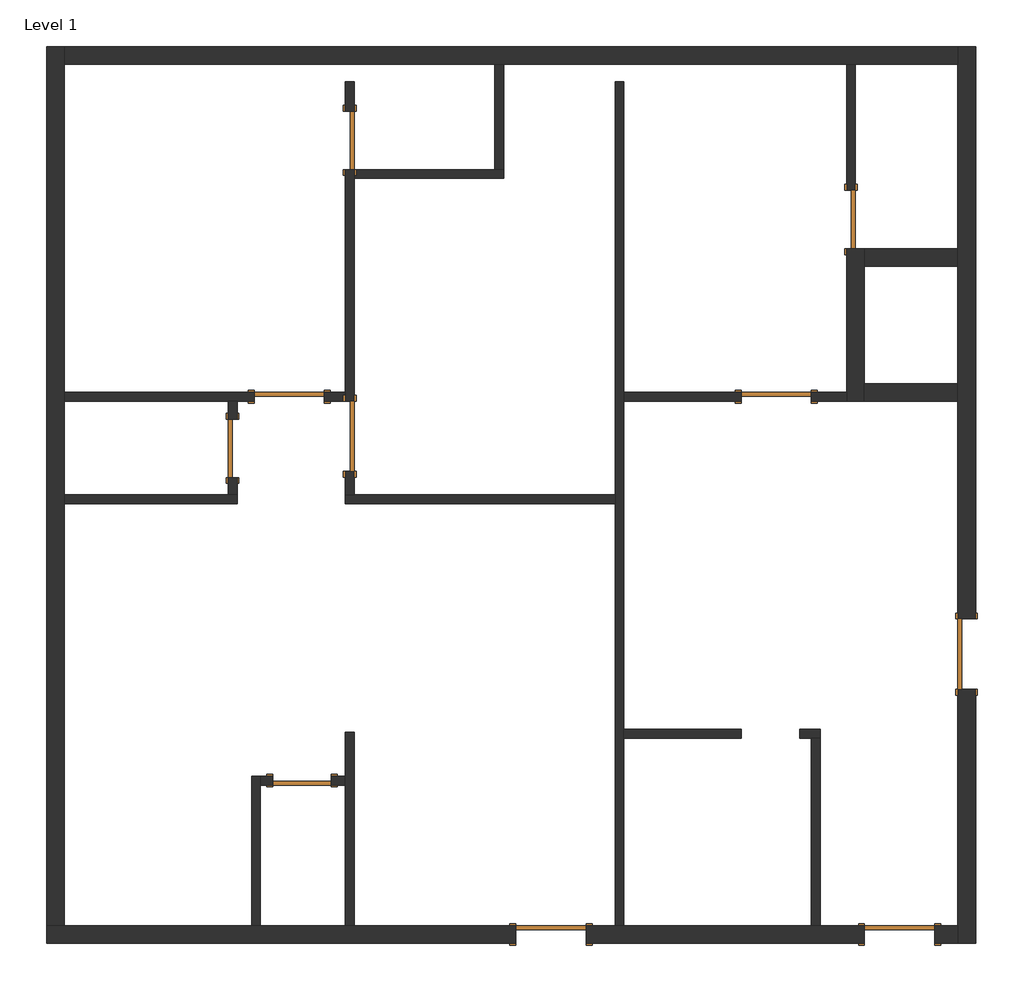
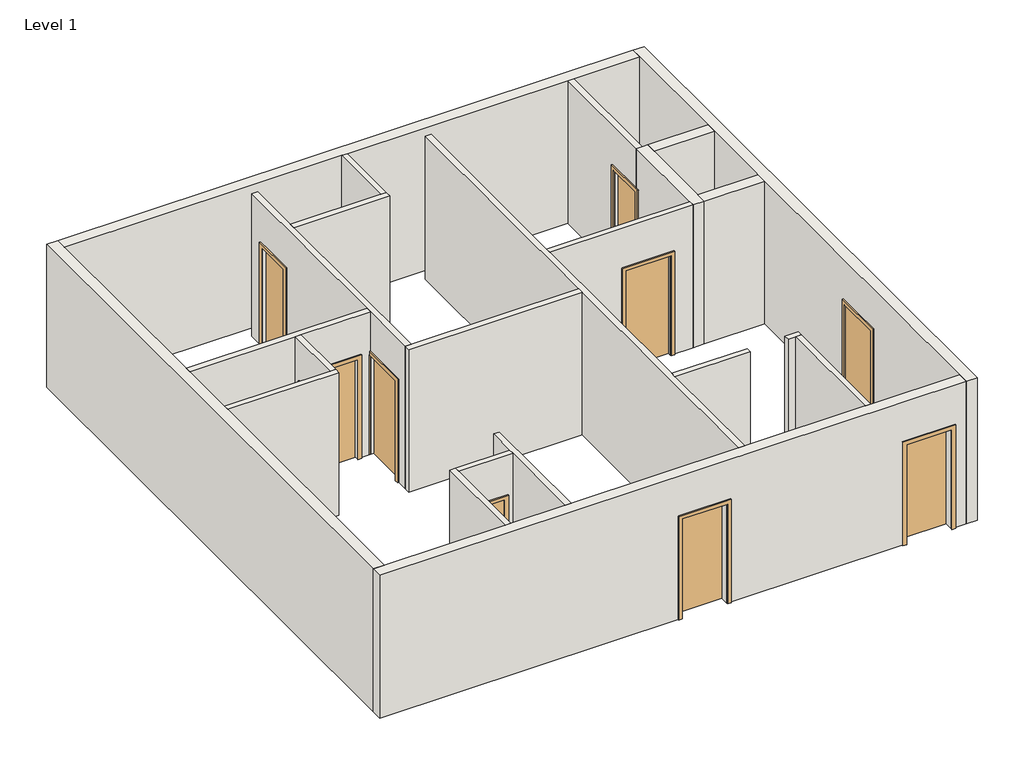
# One storey: 23 walls, 10 doors.
"""IFC4 building model written with IfcOpenShell, lengths in millimetres."""

from ifc_helpers import new_model, si_unit, frame, origin, origin_with_axes, place, context, project, spatial, polyline, outline, extrude, faceted_brep, transform, mapped, element, save
from components import door_214872d5, door_78caadf7, door_e5f9f3c4, door_0ca8825f, door_a90ba1ad

model = new_model("IFC4")

# Units and contexts
model_context = context("Model", 3, world=origin())
ifc_project = project(units=[si_unit("LENGTHUNIT", "METRE", prefix="MILLI")], contexts=[model_context])

# Site, building, storey
site = spatial("IfcSite", under=ifc_project)
building = spatial("IfcBuilding", under=site)
storey = spatial("IfcBuildingStorey", under=building, Name="Level 1", Elevation=0.0)

# Doors
placement = place(None, origin())
door_shape = door_214872d5(model_context)
element("IfcDoor", 1, ObjectType="Single-Flush : 30\" x 84\"", at=placement, inside=storey, context=model_context, shape_type="MappedRepresentation", body=[
    mapped(door_shape, transform((-4308.2802303, 5667.3877739, 0.0), x_axis=(0.0, -1.0, 0.0), y_axis=(1.0, 0.0, 0.0), z_axis=(0.0, 0.0, 1.0))),
])
element("IfcDoor", 2, ObjectType="Single-Flush : 30\" x 84\"", at=placement, inside=storey, context=model_context, shape_type="MappedRepresentation", body=[
    mapped(door_shape, transform((2206.8197697, 4638.6877739, 0.0), x_axis=(0.0, -1.0, 0.0), y_axis=(1.0, 0.0, 0.0), z_axis=(0.0, 0.0, 1.0))),
])
element("IfcDoor", 3, ObjectType="Single-Flush : 30\" x 84\"", at=placement, inside=storey, context=model_context, shape_type="MappedRepresentation", body=[
    mapped(door_shape, transform((-5832.2802303, 1662.8764801, 0.0), x_axis=(0.0, 1.0, 0.0), y_axis=(-1.0, 0.0, 0.0), z_axis=(0.0, 0.0, 1.0))),
])
door_2_shape = door_78caadf7(model_context)
element("IfcDoor", 4, ObjectType="Single-Flush : 30\" x 84\"", at=placement, inside=storey, context=model_context, shape_type="MappedRepresentation", body=[
    mapped(door_2_shape, transform((-4929.4173805, -2657.4622261, 0.0), x_axis=(1.0, 0.0, 0.0), y_axis=(0.0, 1.0, 0.0), z_axis=(0.0, 0.0, 1.0))),
])
door_3_shape = door_e5f9f3c4(model_context)
element("IfcDoor", 5, ObjectType="Single-Flush : 36\" x 84\"", at=placement, inside=storey, context=model_context, shape_type="MappedRepresentation", body=[
    mapped(door_3_shape, transform((-5096.3129519, 2333.6377739, 0.0), x_axis=(1.0, 0.0, 0.0), y_axis=(0.0, 1.0, 0.0), z_axis=(0.0, 0.0, 1.0))),
])
element("IfcDoor", 6, ObjectType="Single-Flush : 36\" x 84\"", at=placement, inside=storey, context=model_context, shape_type="MappedRepresentation", body=[
    mapped(door_3_shape, transform((-4308.2802303, 1819.2877739, 0.0), x_axis=(0.0, -1.0, 0.0), y_axis=(1.0, 0.0, 0.0), z_axis=(0.0, 0.0, 1.0))),
])
element("IfcDoor", 7, ObjectType="Single-Flush : 36\" x 84\"", at=placement, inside=storey, context=model_context, shape_type="MappedRepresentation", body=[
    mapped(door_3_shape, transform((1235.2697697, 2333.6377739, 0.0), x_axis=(1.0, 0.0, 0.0), y_axis=(0.0, 1.0, 0.0), z_axis=(0.0, 0.0, 1.0))),
])
door_4_shape = door_0ca8825f(model_context)
element("IfcDoor", 8, ObjectType="Single-Flush : 36\" x 84\"", at=placement, inside=storey, context=model_context, shape_type="MappedRepresentation", body=[
    mapped(door_4_shape, transform((2839.8620702, -4657.7122261, 0.0), x_axis=(1.0, 0.0, 0.0), y_axis=(0.0, 1.0, 0.0), z_axis=(0.0, 0.0, 1.0))),
])
element("IfcDoor", 9, ObjectType="Single-Flush : 36\" x 84\"", at=placement, inside=storey, context=model_context, shape_type="MappedRepresentation", body=[
    mapped(door_4_shape, transform((-1692.7716329, -4657.7122261, 0.0), x_axis=(1.0, 0.0, 0.0), y_axis=(0.0, 1.0, 0.0), z_axis=(0.0, 0.0, 1.0))),
])
door_5_shape = door_a90ba1ad(model_context)
element("IfcDoor", 10, ObjectType="Single-Flush : 36\" x 84\"", at=placement, inside=storey, context=model_context, shape_type="MappedRepresentation", body=[
    mapped(door_5_shape, transform((3711.7697697, -1012.8122261, 0.0), x_axis=(0.0, -1.0, 0.0), y_axis=(1.0, 0.0, 0.0), z_axis=(0.0, 0.0, 1.0))),
])

# Walls
element("IfcWall", 11, ObjectType="Generic - 4.5\"", at=placement, inside=storey, context=model_context, shape_type="Brep", body=[
    faceted_brep([(-4639.1129519, 2276.4877739, 2133.6), (-4639.1129519, 2276.4877739, 0.0), (-4365.4302303, 2276.4877739, 0.0), (-4365.4302303, 2276.4877739, 3048.0), (-5775.1302303, 2276.4877739, 3048.0), (-5889.4302303, 2276.4877739, 3048.0), (-8023.0302303, 2276.4877739, 3048.0), (-8023.0302303, 2276.4877739, 0.0), (-5889.4302303, 2276.4877739, 0.0), (-5775.1302303, 2276.4877739, 0.0), (-5553.5129519, 2276.4877739, 0.0), (-5553.5129519, 2276.4877739, 2133.6), (-4365.4302303, 2390.7877739, 0.0), (-4639.1129519, 2390.7877739, 0.0), (-4639.1129519, 2390.7877739, 2133.6), (-5553.5129519, 2390.7877739, 2133.6), (-5553.5129519, 2390.7877739, 0.0), (-8023.0302303, 2390.7877739, 0.0), (-8023.0302303, 2390.7877739, 3048.0), (-4365.4302303, 2390.7877739, 3048.0)], [[[0, 1, 2, 3, 4, 5, 6, 7, 8, 9, 10, 11]], [[12, 13, 14, 15, 16, 17, 18, 19]], [[2, 1, 13, 12]], [[10, 9, 8, 7, 17, 16]], [[6, 5, 4, 3, 19, 18]], [[7, 6, 18, 17]], [[3, 2, 12, 19]], [[14, 13, 1, 0]], [[15, 14, 0, 11]], [[16, 15, 11, 10]]]),
])
element("IfcWall", 12, ObjectType="Generic - 4.5\"", at=placement, inside=storey, context=model_context, shape_type="Brep", body=[
    faceted_brep([(-4251.1302303, 2276.4877739, 0.0), (-4251.1302303, 5172.0877739, 0.0), (-4251.1302303, 5286.3877739, 0.0), (-4251.1302303, 5286.3877739, 2133.6), (-4251.1302303, 6048.3877739, 2133.6), (-4251.1302303, 6048.3877739, 0.0), (-4251.1302303, 6429.3877739, 0.0), (-4251.1302303, 6429.3877739, 3048.0), (-4251.1302303, 5286.3877739, 3048.0), (-4251.1302303, 5172.0877739, 3048.0), (-4251.1302303, 1057.2877739, 3048.0), (-4251.1302303, 1057.2877739, 0.0), (-4251.1302303, 1362.0877739, 0.0), (-4251.1302303, 1362.0877739, 2133.6), (-4251.1302303, 2276.4877739, 2133.6), (-4365.4302303, 5286.3877739, 2133.6), (-4365.4302303, 5286.3877739, 0.0), (-4365.4302303, 2390.7877739, 0.0), (-4365.4302303, 2276.4877739, 0.0), (-4365.4302303, 2276.4877739, 2133.6), (-4365.4302303, 1362.0877739, 2133.6), (-4365.4302303, 1362.0877739, 0.0), (-4365.4302303, 1057.2877739, 0.0), (-4365.4302303, 1057.2877739, 3048.0), (-4365.4302303, 2276.4877739, 3048.0), (-4365.4302303, 2390.7877739, 3048.0), (-4365.4302303, 6429.3877739, 3048.0), (-4365.4302303, 6429.3877739, 0.0), (-4365.4302303, 6048.3877739, 0.0), (-4365.4302303, 6048.3877739, 2133.6)], [[[0, 1, 2, 3, 4, 5, 6, 7, 8, 9, 10, 11, 12, 13, 14]], [[15, 16, 17, 18, 19, 20, 21, 22, 23, 24, 25, 26, 27, 28, 29]], [[22, 21, 12, 11]], [[28, 27, 6, 5]], [[18, 17, 16, 2, 1, 0]], [[7, 6, 27, 26]], [[10, 9, 8, 7, 26, 25, 24, 23]], [[11, 10, 23, 22]], [[13, 12, 21, 20]], [[14, 13, 20, 19]], [[0, 14, 19, 18]], [[3, 2, 16, 15]], [[4, 3, 15, 29]], [[5, 4, 29, 28]]]),
])
element("IfcWall", 13, ObjectType="Generic - 4.5\"", at=placement, inside=storey, context=model_context, shape_type="Brep", body=[
    faceted_brep([(-4251.1302303, 5172.0877739, 0.0), (-2308.0302303, 5172.0877739, 0.0), (-2308.0302303, 5172.0877739, 3048.0), (-4251.1302303, 5172.0877739, 3048.0), (-4251.1302303, 5286.3877739, 0.0), (-4251.1302303, 5286.3877739, 3048.0), (-2422.3302303, 5286.3877739, 3048.0), (-2308.0302303, 5286.3877739, 3048.0), (-2308.0302303, 5286.3877739, 0.0), (-2422.3302303, 5286.3877739, 0.0)], [[[0, 1, 2, 3]], [[4, 5, 6, 7, 8, 9]], [[1, 0, 4, 9, 8]], [[3, 2, 7, 6, 5]], [[2, 1, 8, 7]], [[0, 3, 5, 4]]]),
])
element("IfcWall", 14, ObjectType="Generic - 4.5\"", at=placement, inside=storey, context=model_context, shape_type="SweptSolid", body=[
    extrude(outline(polyline([(-2308.0302303, 6657.9877739), (-2308.0302303, 5286.3877739), (-2422.3302303, 5286.3877739), (-2422.3302303, 6657.9877739), (-2308.0302303, 6657.9877739)])), origin_with_axes(), (0.0, 0.0, 1.0), 3048.0),
])
element("IfcWall", 15, ObjectType="Generic - 4.5\"", at=placement, inside=storey, context=model_context, shape_type="SweptSolid", body=[
    extrude(outline(polyline([(4257.6877739, 3048.0), (6657.9877739, 3048.0), (6657.9877739, 0.0), (5019.6877739, 0.0), (5019.6877739, 2133.6), (4257.6877739, 2133.6), (4257.6877739, 3048.0)])), frame((2149.6697697, 0.0, 0.0), z_axis=(1.0, 0.0, 0.0), x_axis=(0.0, 1.0, 0.0)), (0.0, 0.0, 1.0), 114.3),
])
element("IfcWall", 16, ObjectType="Generic - 4.5\"", at=placement, inside=storey, context=model_context, shape_type="Brep", body=[
    faceted_brep([(-5470.3302303, -4543.4122261, 0.0), (-5470.3302303, -2714.6122261, 0.0), (-5470.3302303, -2600.3122261, 0.0), (-5470.3302303, -2600.3122261, 3048.0), (-5470.3302303, -2714.6122261, 3048.0), (-5470.3302303, -4543.4122261, 3048.0), (-5584.6302303, -4543.4122261, 0.0), (-5584.6302303, -4543.4122261, 3048.0), (-5584.6302303, -2600.3122261, 3048.0), (-5584.6302303, -2600.3122261, 0.0)], [[[0, 1, 2, 3, 4, 5]], [[6, 7, 8, 9]], [[2, 1, 0, 6, 9]], [[5, 4, 3, 8, 7]], [[0, 5, 7, 6]], [[3, 2, 9, 8]]]),
])
element("IfcWall", 17, ObjectType="Generic - 4.5\"", at=placement, inside=storey, context=model_context, shape_type="SweptSolid", body=[
    extrude(outline(polyline([(2133.6, -4548.4173805), (0.0, -4548.4173805), (0.0, -4365.4302303), (3048.0, -4365.4302303), (3048.0, -5470.3302303), (0.0, -5470.3302303), (0.0, -5310.4173805), (2133.6, -5310.4173805), (2133.6, -4548.4173805)])), frame((0.0, -2714.6122261, 0.0), z_axis=(0.0, 1.0, 0.0), x_axis=(0.0, 0.0, 1.0)), (0.0, 0.0, 1.0), 114.3),
])
element("IfcWall", 18, ObjectType="Generic - 4.5\"", at=placement, inside=storey, context=model_context, shape_type="Brep", body=[
    faceted_brep([(-4251.1302303, -4543.4122261, 0.0), (-4251.1302303, -2028.8122261, 0.0), (-4251.1302303, -2028.8122261, 3048.0), (-4251.1302303, -4543.4122261, 3048.0), (-4365.4302303, -4543.4122261, 0.0), (-4365.4302303, -4543.4122261, 3048.0), (-4365.4302303, -2714.6122261, 3048.0), (-4365.4302303, -2600.3122261, 3048.0), (-4365.4302303, -2028.8122261, 3048.0), (-4365.4302303, -2028.8122261, 0.0), (-4365.4302303, -2600.3122261, 0.0), (-4365.4302303, -2714.6122261, 0.0)], [[[0, 1, 2, 3]], [[4, 5, 6, 7, 8, 9, 10, 11]], [[1, 0, 4, 11, 10, 9]], [[2, 1, 9, 8]], [[3, 2, 8, 7, 6, 5]], [[0, 3, 5, 4]]]),
])
element("IfcWall", 19, ObjectType="Generic - 4.5\"", at=placement, inside=storey, context=model_context, shape_type="Brep", body=[
    faceted_brep([(-745.9302303, -4543.4122261, 0.0), (-745.9302303, -2105.0122261, 0.0), (-745.9302303, -1990.7122261, 0.0), (-745.9302303, 2276.4877739, 0.0), (-745.9302303, 2390.7877739, 0.0), (-745.9302303, 6429.3877739, 0.0), (-745.9302303, 6429.3877739, 3048.0), (-745.9302303, 2390.7877739, 3048.0), (-745.9302303, 2276.4877739, 3048.0), (-745.9302303, -1990.7122261, 3048.0), (-745.9302303, -2105.0122261, 3048.0), (-745.9302303, -4543.4122261, 3048.0), (-860.2302303, -4543.4122261, 0.0), (-860.2302303, -4543.4122261, 3048.0), (-860.2302303, 942.9877739, 3048.0), (-860.2302303, 1057.2877739, 3048.0), (-860.2302303, 6429.3877739, 3048.0), (-860.2302303, 6429.3877739, 0.0), (-860.2302303, 1057.2877739, 0.0), (-860.2302303, 942.9877739, 0.0)], [[[0, 1, 2, 3, 4, 5, 6, 7, 8, 9, 10, 11]], [[12, 13, 14, 15, 16, 17, 18, 19]], [[5, 4, 3, 2, 1, 0, 12, 19, 18, 17]], [[6, 5, 17, 16]], [[11, 10, 9, 8, 7, 6, 16, 15, 14, 13]], [[0, 11, 13, 12]]]),
])
element("IfcWall", 20, ObjectType="Generic - 4.5\"", at=placement, inside=storey, context=model_context, shape_type="SweptSolid", body=[
    extrude(outline(polyline([(2133.6, 1692.4697697), (0.0, 1692.4697697), (0.0, 2149.6697697), (3048.0, 2149.6697697), (3048.0, -745.9302303), (0.0, -745.9302303), (0.0, 778.0697697), (2133.6, 778.0697697), (2133.6, 1692.4697697)])), frame((0.0, 2276.4877739, 0.0), z_axis=(0.0, 1.0, 0.0), x_axis=(0.0, 0.0, 1.0)), (0.0, 0.0, 1.0), 114.3),
])
element("IfcWall", 21, ObjectType="Generic - 4.5\"", at=placement, inside=storey, context=model_context, shape_type="Brep", body=[
    faceted_brep([(1540.0697697, -2105.0122261, 0.0), (1692.4697697, -2105.0122261, 0.0), (1806.7697697, -2105.0122261, 0.0), (1806.7697697, -2105.0122261, 3048.0), (1692.4697697, -2105.0122261, 3048.0), (1540.0697697, -2105.0122261, 3048.0), (1540.0697697, -1990.7122261, 0.0), (1540.0697697, -1990.7122261, 3048.0), (1806.7697697, -1990.7122261, 3048.0), (1806.7697697, -1990.7122261, 0.0)], [[[0, 1, 2, 3, 4, 5]], [[6, 7, 8, 9]], [[2, 1, 0, 6, 9]], [[5, 4, 3, 8, 7]], [[0, 5, 7, 6]], [[3, 2, 9, 8]]]),
])
element("IfcWall", 22, ObjectType="Generic - 4.5\"", at=placement, inside=storey, context=model_context, shape_type="SweptSolid", body=[
    extrude(outline(polyline([(1692.4697697, -4543.4122261), (1692.4697697, -2105.0122261), (1806.7697697, -2105.0122261), (1806.7697697, -4543.4122261), (1692.4697697, -4543.4122261)])), origin_with_axes(), (0.0, 0.0, 1.0), 3048.0),
])
element("IfcWall", 23, ObjectType="Generic - 4.5\"", at=placement, inside=storey, context=model_context, shape_type="SweptSolid", body=[
    extrude(outline(polyline([(-745.9302303, -1990.7122261), (778.0697697, -1990.7122261), (778.0697697, -2105.0122261), (-745.9302303, -2105.0122261), (-745.9302303, -1990.7122261)])), origin_with_axes(), (0.0, 0.0, 1.0), 3048.0),
])
element("IfcWall", 24, ObjectType="Generic - 4.5\"", at=placement, inside=storey, context=model_context, shape_type="Brep", body=[
    faceted_brep([(-860.2302303, 1057.2877739, 0.0), (-4251.1302303, 1057.2877739, 0.0), (-4365.4302303, 1057.2877739, 0.0), (-4365.4302303, 1057.2877739, 3048.0), (-4251.1302303, 1057.2877739, 3048.0), (-860.2302303, 1057.2877739, 3048.0), (-860.2302303, 942.9877739, 0.0), (-860.2302303, 942.9877739, 3048.0), (-4365.4302303, 942.9877739, 3048.0), (-4365.4302303, 942.9877739, 0.0)], [[[0, 1, 2, 3, 4, 5]], [[6, 7, 8, 9]], [[2, 1, 0, 6, 9]], [[3, 2, 9, 8]], [[5, 4, 3, 8, 7]], [[0, 5, 7, 6]]]),
])
element("IfcWall", 25, ObjectType="Generic - 4.5\"", at=placement, inside=storey, context=model_context, shape_type="Brep", body=[
    faceted_brep([(-8023.0302303, 942.9877739, 0.0), (-5775.1302303, 942.9877739, 0.0), (-5775.1302303, 942.9877739, 3048.0), (-8023.0302303, 942.9877739, 3048.0), (-8023.0302303, 1057.2877739, 0.0), (-8023.0302303, 1057.2877739, 3048.0), (-5889.4302303, 1057.2877739, 3048.0), (-5775.1302303, 1057.2877739, 3048.0), (-5775.1302303, 1057.2877739, 0.0), (-5889.4302303, 1057.2877739, 0.0)], [[[0, 1, 2, 3]], [[4, 5, 6, 7, 8, 9]], [[1, 0, 4, 9, 8]], [[3, 2, 7, 6, 5]], [[0, 3, 5, 4]], [[2, 1, 8, 7]]]),
])
element("IfcWall", 26, ObjectType="Generic - 4.5\"", at=placement, inside=storey, context=model_context, shape_type="SweptSolid", body=[
    extrude(outline(polyline([(2276.4877739, 0.0), (2043.8764801, 0.0), (2043.8764801, 2133.6), (1281.8764801, 2133.6), (1281.8764801, 0.0), (1057.2877739, 0.0), (1057.2877739, 3048.0), (2276.4877739, 3048.0), (2276.4877739, 0.0)])), frame((-5889.4302303, 0.0, 0.0), z_axis=(1.0, 0.0, 0.0), x_axis=(0.0, 1.0, 0.0)), (0.0, 0.0, 1.0), 114.3),
])
element("IfcWall", 27, ObjectType="Generic - 9\"", at=placement, inside=storey, context=model_context, shape_type="Brep", body=[
    faceted_brep([(3597.4697697, -1470.0122261, 2133.6), (3597.4697697, -1470.0122261, 0.0), (3597.4697697, -4543.4122261, 0.0), (3597.4697697, -4772.0122261, 0.0), (3597.4697697, -4772.0122261, 3048.0), (3597.4697697, -4543.4122261, 3048.0), (3597.4697697, 2276.4877739, 3048.0), (3597.4697697, 2505.0877739, 3048.0), (3597.4697697, 4029.0877739, 3048.0), (3597.4697697, 4257.6877739, 3048.0), (3597.4697697, 6657.9877739, 3048.0), (3597.4697697, 6886.5877739, 3048.0), (3597.4697697, 6886.5877739, 0.0), (3597.4697697, 6657.9877739, 0.0), (3597.4697697, 4257.6877739, 0.0), (3597.4697697, 4029.0877739, 0.0), (3597.4697697, 2505.0877739, 0.0), (3597.4697697, 2276.4877739, 0.0), (3597.4697697, -555.6122261, 0.0), (3597.4697697, -555.6122261, 2133.6), (3826.0697697, -4772.0122261, 0.0), (3826.0697697, -1470.0122261, 0.0), (3826.0697697, -1470.0122261, 2133.6), (3826.0697697, -555.6122261, 2133.6), (3826.0697697, -555.6122261, 0.0), (3826.0697697, 6886.5877739, 0.0), (3826.0697697, 6886.5877739, 3048.0), (3826.0697697, -4772.0122261, 3048.0)], [[[0, 1, 2, 3, 4, 5, 6, 7, 8, 9, 10, 11, 12, 13, 14, 15, 16, 17, 18, 19]], [[20, 21, 22, 23, 24, 25, 26, 27]], [[3, 2, 1, 21, 20]], [[18, 17, 16, 15, 14, 13, 12, 25, 24]], [[11, 10, 9, 8, 7, 6, 5, 4, 27, 26]], [[4, 3, 20, 27]], [[12, 11, 26, 25]], [[22, 21, 1, 0]], [[23, 22, 0, 19]], [[24, 23, 19, 18]]]),
])
element("IfcWall", 28, ObjectType="Generic - 9\"", at=placement, inside=storey, context=model_context, shape_type="Brep", body=[
    faceted_brep([(2382.6620702, -4543.4122261, 0.0), (1806.7697697, -4543.4122261, 0.0), (1692.4697697, -4543.4122261, 0.0), (-745.9302303, -4543.4122261, 0.0), (-860.2302303, -4543.4122261, 0.0), (-1235.5716329, -4543.4122261, 0.0), (-1235.5716329, -4543.4122261, 2133.6), (-2149.9716329, -4543.4122261, 2133.6), (-2149.9716329, -4543.4122261, 0.0), (-4251.1302303, -4543.4122261, 0.0), (-4365.4302303, -4543.4122261, 0.0), (-5470.3302303, -4543.4122261, 0.0), (-5584.6302303, -4543.4122261, 0.0), (-8023.0302303, -4543.4122261, 0.0), (-8251.6302303, -4543.4122261, 0.0), (-8251.6302303, -4543.4122261, 3048.0), (-8023.0302303, -4543.4122261, 3048.0), (-5584.6302303, -4543.4122261, 3048.0), (-5470.3302303, -4543.4122261, 3048.0), (-4365.4302303, -4543.4122261, 3048.0), (-4251.1302303, -4543.4122261, 3048.0), (-860.2302303, -4543.4122261, 3048.0), (-745.9302303, -4543.4122261, 3048.0), (1692.4697697, -4543.4122261, 3048.0), (1806.7697697, -4543.4122261, 3048.0), (3597.4697697, -4543.4122261, 3048.0), (3597.4697697, -4543.4122261, 0.0), (3297.0620702, -4543.4122261, 0.0), (3297.0620702, -4543.4122261, 2133.6), (2382.6620702, -4543.4122261, 2133.6), (-1235.5716329, -4772.0122261, 2133.6), (-1235.5716329, -4772.0122261, 0.0), (2382.6620702, -4772.0122261, 0.0), (2382.6620702, -4772.0122261, 2133.6), (3297.0620702, -4772.0122261, 2133.6), (3297.0620702, -4772.0122261, 0.0), (3597.4697697, -4772.0122261, 0.0), (3597.4697697, -4772.0122261, 3048.0), (-8251.6302303, -4772.0122261, 3048.0), (-8251.6302303, -4772.0122261, 0.0), (-2149.9716329, -4772.0122261, 0.0), (-2149.9716329, -4772.0122261, 2133.6)], [[[0, 1, 2, 3, 4, 5, 6, 7, 8, 9, 10, 11, 12, 13, 14, 15, 16, 17, 18, 19, 20, 21, 22, 23, 24, 25, 26, 27, 28, 29]], [[30, 31, 32, 33, 34, 35, 36, 37, 38, 39, 40, 41]], [[36, 35, 27, 26]], [[40, 39, 14, 13, 12, 11, 10, 9, 8]], [[32, 31, 5, 4, 3, 2, 1, 0]], [[25, 24, 23, 22, 21, 20, 19, 18, 17, 16, 15, 38, 37]], [[26, 25, 37, 36]], [[15, 14, 39, 38]], [[28, 27, 35, 34]], [[29, 28, 34, 33]], [[0, 29, 33, 32]], [[6, 5, 31, 30]], [[7, 6, 30, 41]], [[8, 7, 41, 40]]]),
])
element("IfcWall", 29, ObjectType="Generic - 9\"", at=placement, inside=storey, context=model_context, shape_type="Brep", body=[
    faceted_brep([(-8023.0302303, -4543.4122261, 0.0), (-8023.0302303, 942.9877739, 0.0), (-8023.0302303, 1057.2877739, 0.0), (-8023.0302303, 2276.4877739, 0.0), (-8023.0302303, 2390.7877739, 0.0), (-8023.0302303, 6657.9877739, 0.0), (-8023.0302303, 6886.5877739, 0.0), (-8023.0302303, 6886.5877739, 3048.0), (-8023.0302303, 6657.9877739, 3048.0), (-8023.0302303, 2390.7877739, 3048.0), (-8023.0302303, 2276.4877739, 3048.0), (-8023.0302303, 1057.2877739, 3048.0), (-8023.0302303, 942.9877739, 3048.0), (-8023.0302303, -4543.4122261, 3048.0), (-8251.6302303, -4543.4122261, 0.0), (-8251.6302303, -4543.4122261, 3048.0), (-8251.6302303, 6886.5877739, 3048.0), (-8251.6302303, 6886.5877739, 0.0)], [[[0, 1, 2, 3, 4, 5, 6, 7, 8, 9, 10, 11, 12, 13]], [[14, 15, 16, 17]], [[6, 5, 4, 3, 2, 1, 0, 14, 17]], [[13, 12, 11, 10, 9, 8, 7, 16, 15]], [[0, 13, 15, 14]], [[7, 6, 17, 16]]]),
])
element("IfcWall", 30, ObjectType="Generic - 9\"", at=placement, inside=storey, context=model_context, shape_type="Brep", body=[
    faceted_brep([(-8023.0302303, 6657.9877739, 0.0), (-2422.3302303, 6657.9877739, 0.0), (-2308.0302303, 6657.9877739, 0.0), (2149.6697697, 6657.9877739, 0.0), (2263.9697697, 6657.9877739, 0.0), (3597.4697697, 6657.9877739, 0.0), (3597.4697697, 6657.9877739, 3048.0), (2263.9697697, 6657.9877739, 3048.0), (2149.6697697, 6657.9877739, 3048.0), (-2308.0302303, 6657.9877739, 3048.0), (-2422.3302303, 6657.9877739, 3048.0), (-8023.0302303, 6657.9877739, 3048.0), (-8023.0302303, 6886.5877739, 0.0), (-8023.0302303, 6886.5877739, 3048.0), (3597.4697697, 6886.5877739, 3048.0), (3597.4697697, 6886.5877739, 0.0)], [[[0, 1, 2, 3, 4, 5, 6, 7, 8, 9, 10, 11]], [[12, 13, 14, 15]], [[5, 4, 3, 2, 1, 0, 12, 15]], [[11, 10, 9, 8, 7, 6, 14, 13]], [[0, 11, 13, 12]], [[6, 5, 15, 14]]]),
])
element("IfcWall", 31, ObjectType="Generic - 9\"", at=placement, inside=storey, context=model_context, shape_type="SweptSolid", body=[
    extrude(outline(polyline([(2378.2697697, 4257.6877739), (3597.4697697, 4257.6877739), (3597.4697697, 4029.0877739), (2378.2697697, 4029.0877739), (2378.2697697, 4257.6877739)])), origin_with_axes(), (0.0, 0.0, 1.0), 3048.0),
])
element("IfcWall", 32, ObjectType="Generic - 9\"", at=placement, inside=storey, context=model_context, shape_type="Brep", body=[
    faceted_brep([(2149.6697697, 4257.6877739, 0.0), (2149.6697697, 2390.7877739, 0.0), (2149.6697697, 2276.4877739, 0.0), (2149.6697697, 2276.4877739, 3048.0), (2149.6697697, 2390.7877739, 3048.0), (2149.6697697, 4257.6877739, 3048.0), (2149.6697697, 4257.6877739, 2133.6), (2378.2697697, 4257.6877739, 0.0), (2378.2697697, 4257.6877739, 3048.0), (2378.2697697, 4029.0877739, 3048.0), (2378.2697697, 2505.0877739, 3048.0), (2378.2697697, 2276.4877739, 3048.0), (2378.2697697, 2276.4877739, 0.0), (2378.2697697, 2505.0877739, 0.0), (2378.2697697, 4029.0877739, 0.0), (2263.9697697, 4257.6877739, 3048.0)], [[[0, 1, 2, 3, 4, 5, 6]], [[7, 8, 9, 10, 11, 12, 13, 14]], [[2, 1, 0, 7, 14, 13, 12]], [[5, 4, 3, 11, 10, 9, 8, 15]], [[0, 6, 5, 15, 8, 7]], [[3, 2, 12, 11]]]),
])
element("IfcWall", 33, ObjectType="Generic - 9\"", at=placement, inside=storey, context=model_context, shape_type="SweptSolid", body=[
    extrude(outline(polyline([(3597.4697697, 2276.4877739), (2378.2697697, 2276.4877739), (2378.2697697, 2505.0877739), (3597.4697697, 2505.0877739), (3597.4697697, 2276.4877739)])), origin_with_axes(), (0.0, 0.0, 1.0), 3048.0),
])

save(model, "model.ifc")

# Revit data of these elements
# Type "Single-Flush : 30\" x 84\""
#   Type Mark = "4"
#   Construction Type Id = "MDOOR"
#   Assembly Code = "C1020"
#   Analytic Construction = "Metal"
#   Thickness = 0' - 2"
#   Heat Transfer Coefficient (U) = 0.651978 BTU/(h·ft²·°F)
#   Height = 7' - 0"
#   Trim Projection Ext = 0' - 1"
#   Trim Projection Int = 0' - 1"
#   Trim Width = 0' - 3"
#   Width = 2' - 6"
#   Define Thermal Properties by = 1
#   Define Thermal Properties by = 1
#   Door Material = Door - Panel
#   Frame Material = Door - Frame
#   Visual Light Transmittance = 0
#   Solar Heat Gain Coefficient = 0
#   Function = (empty or 0)
#   Wall Closure = (empty or 0)
# Type "Single-Flush : 36\" x 84\""
#   Type Mark = "1"
#   Construction Type Id = "MDOOR"
#   Assembly Code = "C1020"
#   Analytic Construction = "Metal"
#   Thickness = 0' - 2"
#   Heat Transfer Coefficient (U) = 0.651978 BTU/(h·ft²·°F)
#   Height = 7' - 0"
#   Trim Projection Ext = 0' - 1"
#   Trim Projection Int = 0' - 1"
#   Trim Width = 0' - 3"
#   Width = 3' - 0"
#   Define Thermal Properties by = 1
#   Define Thermal Properties by = 1
#   Door Material = Door - Panel
#   Frame Material = Door - Frame
#   Visual Light Transmittance = 0
#   Solar Heat Gain Coefficient = 0
#   Function = (empty or 0)
#   Wall Closure = (empty or 0)
# Type "Generic - 4.5\""
#   Assembly Code = "B2010"
#   Layers, outside or top first: 0' - 4 1/2" no material (function 1)
# Type "Generic - 9\""
#   Assembly Code = "B2010"
#   Layers, outside or top first: 0' - 9" no material (function 1)
# Elements 1, 2, 3, 4 (IfcDoor, "Single-Flush : 30\" x 84\"")
#   Phase Created = New Construction
#   Materials on its faces: "Door - Frame", "Door - Panel"
# Elements 5, 6, 7, 8, 9, 10 (IfcDoor, "Single-Flush : 36\" x 84\"")
#   Phase Created = New Construction
#   Materials on its faces: "Door - Frame", "Door - Panel"
# Elements 11, 12, 13, 14, 15, 16, 17, 18, 19, 20, 21, 22, 23, 24, 25, 26 (IfcWall, "Generic - 4.5\"")
#   Top Offset = 0' - 0"
#   Base Offset = 0' - 0"
#   wall height = 10' - 0"
#   Phase Created = New Construction
#   Base Constraint = Level 1
#   Top Constraint = Level 2
#   Materials on its faces: "Default Wall"
# Elements 27, 28, 29, 30, 31, 32, 33 (IfcWall, "Generic - 9\"")
#   Top Offset = 0' - 0"
#   Base Offset = 0' - 0"
#   wall height = 10' - 0"
#   Phase Created = New Construction
#   Base Constraint = Level 1
#   Top Constraint = Level 2
#   Materials on its faces: "Default Wall"
# Materials
#   "Door - Panel": class "Wood", colour RGB 210 159 95, transparency 0, Cost = 0
#   "Door - Frame": colour RGB 118 70 51, transparency 0, Cost = 0
#   "Default Wall": colour RGB 128 128 128, transparency 0, Cost = 0
